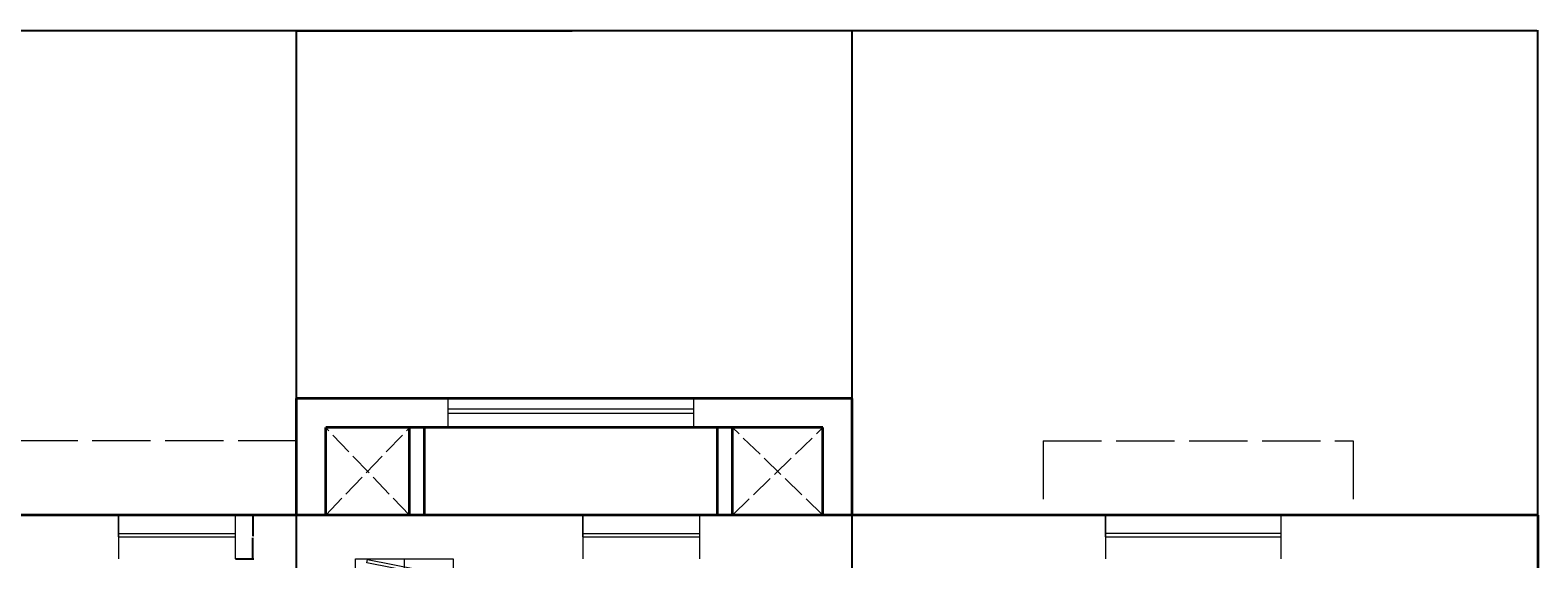
# Model space of a CAD drawing. Units: inches. Extents: x -61 to 1599, y -1316 to 257.
# Tile 204 of 204: x 1213 to 1523, y 149 to 257. Entities that reach past the tile are written whole.
import ezdxf

# ---------------------------------------------------------------- set-up
doc = ezdxf.new("R2010")
doc.units = ezdxf.units.IN
doc.header["$MEASUREMENT"] = 0
doc.linetypes.add('ACAD_ISO02W100', pattern=[15, 12, -3])
for name, color, linetype, lineweight in [('A-ANNO-DIMS', 2, 'Continuous', 18), ('A-FLOR-CASE', 8, 'Continuous', 18), ('A-FLOR-OPEN-HIDN', 8, 'ACAD_ISO02W100', 13), ('A-FLOR-OVHD', 203, 'ACAD_ISO02W100', 13), ('WALLS', 4, 'Continuous', 35), ('WINDOWS', 220, 'Continuous', 18)]:
    doc.layers.add(name, color=color, linetype=linetype, lineweight=lineweight)
doc.styles.get("Standard").update_dxf_attribs({"font": 'arial.ttf'})
doc.dimstyles.get("Standard").update_dxf_attribs({"dimtxt": 0.18, "dimasz": 0.18, "dimexe": 0.18, "dimexo": 0.0625, "dimgap": 0.09, "dimtad": 0, "dimtih": 1, "dimtoh": 1, "dimdec": 0, "dimzin": 0, "dimdsep": 46, "dimlunit": 3, "dimtxsty": 'Standard', "dimcen": 0.09, "dimadec": 0, "dimazin": 0, "dimtfac": 1, "dimtdec": 0, "dimtofl": 0, "dimtmove": 0, "dimatfit": 3, "dimfxl": 1, "dimtolj": 1, "dimtzin": 0, "dimarcsym": 0})

# ---------------------------------------------------------------- blocks, each defined once
blk = doc.blocks.new('WIN-24IN')
for p, q in [((0, 4.5), (0, 9)), ((0, 9), (0, 0)), ((24, 9), (24, 0)), ((0, 5.19), (24, 5.19)), ((0, 4.5), (24, 4.5))]:
    blk.add_line(p, q)
blk = doc.blocks.new('WIN-36IN')
for p, q in [((0, 4.5), (0, 9)), ((0, 9), (0, 0)), ((36, 9), (36, 0)), ((0, 5.26), (36, 5.26)), ((0, 4.5), (36, 4.5)), ((0, 4.5), (36, 4.5))]:
    blk.add_line(p, q)
blk = doc.blocks.new('WIN-51IN')
for p, q in [((0, 0), (0, 6)), ((0, 3.89), (50.52, 3.89)), ((50.52, 0), (50.52, 6)), ((0, 3), (50.52, 3))]:
    blk.add_line(p, q)
blk = doc.blocks.new('WARDROBE-HANGING')
blk.add_line((10.05, 0), (10.05, 68))
for points in [[(20.09, 0), (0, 0), (0, 68), (20.09, 68)], [(2.48, 67.85), (17.75, 64.85), (17.61, 64.14), (2.34, 67.15)], [(1.32, 62.96), (16.59, 59.95), (16.45, 59.25), (1.19, 62.25)], [(1.35, 59.16), (16.22, 63.73), (16.43, 63.04), (1.56, 58.47)], [(1.71, 56.78), (16.98, 53.78), (16.84, 53.07), (1.57, 56.08)], [(1, 46.47), (15.87, 51.04), (16.08, 50.35), (1.21, 45.78)], [(1.39, 50.01), (16.66, 47.01), (16.52, 46.3), (1.26, 49.31)], [(1.36, 44.09), (16.63, 41.09), (16.49, 40.38), (1.23, 43.38)], [(1.26, 37.2), (16.53, 34.2), (16.39, 33.49), (1.12, 36.5)], [(1.28, 33.41), (16.16, 37.98), (16.37, 37.29), (1.49, 32.72)], [(1.65, 31.03), (16.92, 28.03), (16.78, 27.32), (1.51, 30.32)], [(1.26, 25.09), (16.53, 22.09), (16.39, 21.38), (1.12, 24.39)], [(1.28, 21.3), (16.15, 25.87), (16.36, 25.18), (1.49, 20.61)], [(1.65, 18.92), (16.91, 15.92), (16.78, 15.21), (1.51, 18.21)], [(1.91, 13.69), (17.17, 10.68), (17.04, 9.98), (1.77, 12.98)], [(1.93, 9.89), (16.8, 14.46), (17.01, 13.77), (2.14, 9.2)], [(2.29, 7.51), (17.56, 4.51), (17.42, 3.8), (2.16, 6.81)], [(17.49, 1.96), (1.93, 1.96), (1.93, 2.68), (17.49, 2.68)]]:
    blk.add_lwpolyline(points, close=True)
blk = doc.blocks.new('*D615')
at = {"layer": 'A-ANNO-DIMS', "color": 0, "lineweight": -2, "transparency": 16777216}
for p, q in [((1254.94, 157.68), (1258.66, 157.68)), ((1258.48, 157.5), (1258.48, 153.36)), ((1258.48, 148.86), (1258.48, 153)), ((1254.94, 148.68), (1258.66, 148.68))]:
    blk.add_line(p, q, dxfattribs=at)
at = {"layer": 'A-ANNO-DIMS', "color": 0, "transparency": 16777216}
for points in [[(1258.45, 157.5), (1258.51, 157.5), (1258.48, 157.68)], [(1258.45, 148.86), (1258.51, 148.86), (1258.48, 148.68)]]:
    blk.add_solid(points, dxfattribs=at)
at = {"layer": 'DEFPOINTS', "color": 0, "transparency": 16777216}
for p in [(1254.88, 157.68), (1258.48, 157.68), (1254.88, 148.68)]:
    blk.add_point(p, dxfattribs=at)
at = {"layer": 'A-ANNO-DIMS', "color": 0, "transparency": 16777216, "insert": (1258.48, 153.18), "char_height": 0.18, "attachment_point": 5}
blk.add_mtext('\\A1;9 TYP.', dxfattribs=at)
blk = doc.blocks.new('*D686')
at = {"layer": 'A-ANNO-DIMS', "color": 0, "lineweight": -2, "transparency": 16777216}
for p, q in [((14.7, 157.74), (14.7, 257.46)), ((1522.7, 157.74), (1522.7, 257.46)), ((14.88, 257.28), (768.35, 257.28)), ((1522.52, 257.28), (769.05, 257.28))]:
    blk.add_line(p, q, dxfattribs=at)
at = {"layer": 'A-ANNO-DIMS', "color": 0, "transparency": 16777216}
for points in [[(14.88, 257.31), (14.88, 257.25), (14.7, 257.28)], [(1522.52, 257.31), (1522.52, 257.25), (1522.7, 257.28)]]:
    blk.add_solid(points, dxfattribs=at)
at = {"layer": 'DEFPOINTS', "color": 0, "transparency": 16777216}
for p in [(1522.7, 257.28), (14.7, 157.68), (1522.7, 157.68)]:
    blk.add_point(p, dxfattribs=at)
at = {"layer": 'A-ANNO-DIMS', "color": 0, "transparency": 16777216, "insert": (768.7, 257.28), "char_height": 0.18, "attachment_point": 5}
blk.add_mtext('\\A1;1508', dxfattribs=at)
blk = doc.blocks.new('*D708')
at = {"layer": 'A-ANNO-DIMS', "color": 0, "lineweight": -2, "transparency": 16777216}
for p, q in [((1267.48, -588.11), (1267.48, 257.46)), ((1381.7, -588.11), (1381.7, 257.46)), ((1267.66, 257.28), (1324.14, 257.28)), ((1381.52, 257.28), (1325.05, 257.28))]:
    blk.add_line(p, q, dxfattribs=at)
at = {"layer": 'A-ANNO-DIMS', "color": 0, "transparency": 16777216}
for points in [[(1267.66, 257.31), (1267.66, 257.25), (1267.48, 257.28)], [(1381.52, 257.31), (1381.52, 257.25), (1381.7, 257.28)]]:
    blk.add_solid(points, dxfattribs=at)
at = {"layer": 'DEFPOINTS', "color": 0, "transparency": 16777216}
for p in [(1381.7, 257.28), (1267.48, -588.17), (1381.7, -588.17)]:
    blk.add_point(p, dxfattribs=at)
at = {"layer": 'A-ANNO-DIMS', "color": 0, "transparency": 16777216, "insert": (1324.59, 257.28), "char_height": 0.18, "attachment_point": 5}
blk.add_mtext('\\A1;114.22', dxfattribs=at)

msp = doc.modelspace()

# ---------------------------------------------------------------- linework, layer by layer
at = {"layer": 'A-FLOR-OPEN-HIDN', "ltscale": 0.4}
for p, q in [((1273.4807, 157.6771), (1290.6819, 175.6771)), ((1290.6819, 157.6771), (1273.4807, 175.6771)), ((1357.1186, 157.6771), (1375.7028, 175.6771)), ((1375.7028, 157.6771), (1357.1186, 175.6771))]:
    msp.add_line(p, q, dxfattribs=at)
at = {"layer": 'A-FLOR-OVHD'}
for p, q in [((1267.4807, 172.9695), (1138.8585, 172.9695)), ((1420.9886, 172.9695), (1420.9886, 157.6771)), ((1420.9886, 172.9695), (1484.76, 172.9695)), ((1484.76, 172.9695), (1484.76, 157.6771))]:
    msp.add_line(p, q, dxfattribs=at)
at = {"layer": 'WALLS'}
for p, q in [((1267.4807, 157.6771), (1267.4807, 181.6771)), ((1381.7028, 181.6771), (1267.4807, 181.6771)), ((1381.7028, 157.6771), (1381.7028, 181.6771)), ((1273.4807, 157.6771), (1273.4807, 175.6771)), ((1375.7028, 175.6771), (1273.4807, 175.6771)), ((1290.6819, 157.6771), (1290.6819, 175.6771)), ((1293.7747, 157.6771), (1293.7747, 175.6771)), ((1354.0257, 157.6771), (1354.0257, 175.6771)), ((1357.1186, 157.6771), (1357.1186, 175.6771)), ((1375.7028, 157.6771), (1375.7028, 175.6771)), ((1522.7028, 157.6771), (992.7028, 157.6771)), ((1522.7028, 157.6771), (1522.7028, 34.831))]:
    msp.add_line(p, q, dxfattribs=at)

# ---------------------------------------------------------------- block references
at = {"layer": 'A-FLOR-CASE'}
msp.add_blockref('WARDROBE-HANGING', (1279.609, 80.677), dxfattribs=at)
at = {"layer": 'WINDOWS'}
for name, p in [('WIN-51IN', (1298.659, 175.677)), ('WIN-24IN', (1230.882, 148.677)), ('WIN-24IN', (1326.3196, 148.677)), ('WIN-36IN', (1433.8326, 148.677))]:
    msp.add_blockref(name, p, dxfattribs=at)

# ---------------------------------------------------------------- dimensions: what is measured, and where the dimension line sits
at = {"layer": 'A-ANNO-DIMS'}
for base, p1, p2, override, picture, middle in [((1522.7028, 257.2771), (14.7028, 157.6771), (1522.7028, 157.6771), {"dimdec": 0, "dimlfac": 1, "dimrnd": 0, "dimzin": 0, "dimdsep": 46, "dimlunit": 2}, '*D686', (768.7028, 257.2771)), ((1381.7028, 257.2771), (1267.4807, -588.169), (1381.7028, -588.169), {"dimdec": 2, "dimlfac": 1, "dimrnd": 0, "dimzin": 0, "dimdsep": 46, "dimlunit": 2}, '*D708', (1324.5917, 257.2771))]:
    dim = msp.add_linear_dim(base=base, p1=p1, p2=p2, dimstyle='Standard', override=override, dxfattribs=at)
    dim.commit()
    dim.dimension.update_dxf_attribs({"geometry": picture, "text_midpoint": middle})
dim = msp.add_linear_dim(base=(1258.4825, 157.6771), p1=(1254.8825, 148.6771), p2=(1254.8825, 157.6771), angle=90, text='<> TYP.', dimstyle='Standard', override={"dimdec": 0, "dimlfac": 1, "dimrnd": 0, "dimzin": 0, "dimdsep": 46, "dimlunit": 2}, dxfattribs=at)
dim.commit()
dim.dimension.update_dxf_attribs({"geometry": '*D615', "text_midpoint": (1258.4825, 153.1771)})

doc.saveas('drawing.dxf')
